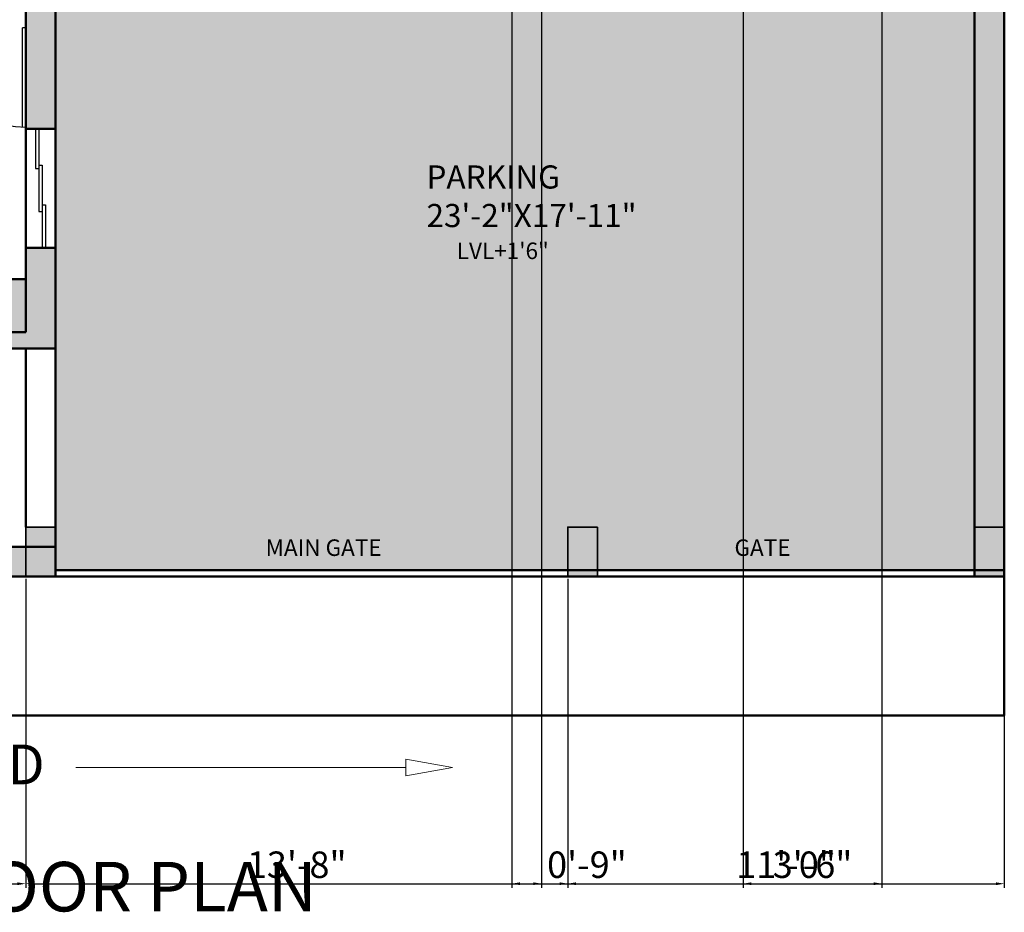
# Model space of a CAD drawing. Units: inches. Extents: x 1770 to 3141, y 984 to 1614.
# Tile 5 of 12: x 2115 to 2413, y 984 to 1254. Entities that reach past the tile are written whole.
import ezdxf

# ---------------------------------------------------------------- set-up
doc = ezdxf.new("R2010")
doc.units = ezdxf.units.IN
for name, color, linetype, lineweight in [('A-ANNO-DIMS', 2, 'Continuous', 18), ('A-ANNO-SYMB', 7, 'Continuous', 18), ('A-ANNO-TEXT', 7, 'Continuous', 18), ('A-AREA-IDEN', 3, 'Continuous', 18), ('A-COLS', 1, 'Continuous', 35), ('A-DOOR', 4, 'Continuous', 25), ('A-FLOR-PATT', 252, 'Continuous', 13), ('A-GLAZ', 5, 'Continuous', 25), ('A-WALL', 7, 'Continuous', 50), ('A-WALL-PATT', 8, 'Continuous', 13)]:
    doc.layers.add(name, color=color, linetype=linetype, lineweight=lineweight)
doc.styles.get("Standard").update_dxf_attribs({"font": 'arial.ttf'})
doc.dimstyles.new('ISO-25', dxfattribs={"dimtxt": 8, "dimasz": 2.5, "dimexe": 1.25, "dimexo": 0.625, "dimtad": 1, "dimdec": 1, "dimlunit": 3, "dimtxsty": 'Standard', "dimcen": 2.5, "dimclrt": 1, "dimadec": 0, "dimazin": 0, "dimtfac": 1, "dimtdec": 1, "dimtmove": 0, "dimatfit": 3, "dimfxl": 1, "dimarcsym": 0})

# ---------------------------------------------------------------- blocks, each defined once
blk = doc.blocks.new("D2 2'6")
for p, q in [((0, 30), (0, 0)), ((1, 30), (1, 0)), ((0, 0), (1, 0))]:
    blk.add_line(p, q)
blk.add_arc((0, 0), 30, 0, 90)
blk = doc.blocks.new('COLUMN-9x15')
at = {"transparency": 33554687}
h = blk.add_hatch(color=256, dxfattribs=at)
h.dxf.hatch_style = 1
h.paths.add_polyline_path([(9, 15), (0, 15), (0, 0), (9, 0)])
blk.add_lwpolyline([(9, 15), (0, 15), (0, 0), (9, 0)], close=True)
blk = doc.blocks.new('*D111')
at = {"layer": 'A-ANNO-DIMS', "color": 0, "lineweight": -2, "transparency": 16777216}
for p, q in [((2001.73, 1084.55), (2001.73, 991.02)), ((2116.73, 1084.55), (2116.73, 991.02)), ((2004.23, 992.27), (2114.23, 992.27))]:
    blk.add_line(p, q, dxfattribs=at)
at = {"layer": 'A-ANNO-DIMS', "color": 0, "transparency": 16777216}
for points in [[(2004.23, 992.69), (2004.23, 991.85), (2001.73, 992.27)], [(2114.23, 992.69), (2114.23, 991.85), (2116.73, 992.27)]]:
    blk.add_solid(points, dxfattribs=at)
at = {"layer": 'Defpoints', "color": 0, "transparency": 16777216}
for p in [(2001.73, 1085.18), (2116.73, 1085.18), (2116.73, 992.27)]:
    blk.add_point(p, dxfattribs=at)
at = {"layer": 'A-ANNO-DIMS', "color": 1, "transparency": 16777216, "insert": (2059.23, 996.98), "char_height": 8, "attachment_point": 5}
blk.add_mtext('9\'-7"', dxfattribs=at)
blk = doc.blocks.new('*D112')
at = {"layer": 'A-ANNO-DIMS', "color": 0, "lineweight": -2, "transparency": 16777216}
for p, q in [((2116.73, 1084.55), (2116.73, 991.02)), ((2280.7, 1084.55), (2280.7, 991.02)), ((2119.23, 992.27), (2278.2, 992.27))]:
    blk.add_line(p, q, dxfattribs=at)
at = {"layer": 'A-ANNO-DIMS', "color": 0, "transparency": 16777216}
for points in [[(2119.23, 992.69), (2119.23, 991.85), (2116.73, 992.27)], [(2278.2, 992.69), (2278.2, 991.85), (2280.7, 992.27)]]:
    blk.add_solid(points, dxfattribs=at)
at = {"layer": 'Defpoints', "color": 0, "transparency": 16777216}
for p in [(2116.73, 1085.18), (2280.7, 1085.18), (2280.7, 992.27)]:
    blk.add_point(p, dxfattribs=at)
at = {"layer": 'A-ANNO-DIMS', "color": 1, "transparency": 16777216, "insert": (2198.71, 996.98), "char_height": 8, "attachment_point": 5}
blk.add_mtext('13\'-8"', dxfattribs=at)
blk = doc.blocks.new('*D113')
at = {"layer": 'A-ANNO-DIMS', "color": 0, "lineweight": -2, "transparency": 16777216}
for p, q in [((2280.7, 1084.55), (2280.7, 991.02)), ((2412.73, 1084.55), (2412.73, 991.02)), ((2283.2, 992.27), (2410.23, 992.27))]:
    blk.add_line(p, q, dxfattribs=at)
at = {"layer": 'A-ANNO-DIMS', "color": 0, "transparency": 16777216}
for points in [[(2283.2, 992.69), (2283.2, 991.85), (2280.7, 992.27)], [(2410.23, 992.69), (2410.23, 991.85), (2412.73, 992.27)]]:
    blk.add_solid(points, dxfattribs=at)
at = {"layer": 'Defpoints', "color": 0, "transparency": 16777216}
for p in [(2280.7, 1085.18), (2412.73, 1085.18), (2412.73, 992.27)]:
    blk.add_point(p, dxfattribs=at)
at = {"layer": 'A-ANNO-DIMS', "color": 1, "transparency": 16777216, "insert": (2346.71, 996.98), "char_height": 8, "attachment_point": 5}
blk.add_mtext('11\'-0"', dxfattribs=at)
blk = doc.blocks.new('*D118')
at = {"layer": 'A-ANNO-DIMS', "color": 0, "lineweight": -2, "transparency": 16777216}
for p, q in [((2272.73, 1355.55), (2272.73, 991.02)), ((2263.73, 1346.55), (2263.73, 991.02)), ((2266.23, 992.27), (2270.23, 992.27)), ((2272.73, 992.27), (2297.75, 992.27))]:
    blk.add_line(p, q, dxfattribs=at)
at = {"layer": 'A-ANNO-DIMS', "color": 0, "transparency": 16777216}
for points in [[(2266.23, 992.69), (2266.23, 991.85), (2263.73, 992.27)], [(2270.23, 992.69), (2270.23, 991.85), (2272.73, 992.27)]]:
    blk.add_solid(points, dxfattribs=at)
at = {"layer": 'Defpoints', "color": 0, "transparency": 16777216}
for p in [(2272.73, 1356.18), (2263.73, 1347.18), (2272.73, 992.27)]:
    blk.add_point(p, dxfattribs=at)
at = {"layer": 'A-ANNO-DIMS', "color": 1, "transparency": 16777216, "insert": (2286.49, 996.98), "char_height": 8, "attachment_point": 5}
blk.add_mtext('0\'-9"', dxfattribs=at)
blk = doc.blocks.new('*D119')
at = {"layer": 'A-ANNO-DIMS', "color": 0, "lineweight": -2, "transparency": 16777216}
for p, q in [((2333.73, 1355.55), (2333.73, 991.02)), ((2375.73, 1346.55), (2375.73, 991.02)), ((2336.23, 992.27), (2373.23, 992.27))]:
    blk.add_line(p, q, dxfattribs=at)
at = {"layer": 'A-ANNO-DIMS', "color": 0, "transparency": 16777216}
for points in [[(2336.23, 992.69), (2336.23, 991.85), (2333.73, 992.27)], [(2373.23, 992.69), (2373.23, 991.85), (2375.73, 992.27)]]:
    blk.add_solid(points, dxfattribs=at)
at = {"layer": 'Defpoints', "color": 0, "transparency": 16777216}
for p in [(2333.73, 1356.18), (2375.73, 1347.18), (2375.73, 992.27)]:
    blk.add_point(p, dxfattribs=at)
at = {"layer": 'A-ANNO-DIMS', "color": 1, "transparency": 16777216, "insert": (2354.73, 996.98), "char_height": 8, "attachment_point": 5}
blk.add_mtext('3\'-6"', dxfattribs=at)

msp = doc.modelspace()

# ---------------------------------------------------------------- hatches: boundary and pattern name
at = {"layer": 'A-FLOR-PATT'}
h = msp.add_hatch(color=256, dxfattribs=at)
h.dxf.hatch_style = 1
h.paths.add_polyline_path([(2403.73, 1288.18), (2239.73, 1288.18), (2239.73, 1300.18), (2193.73, 1300.18), (2193.73, 1288.18), (2125.73, 1288.18), (2125.73, 1154.18), (2125.73, 1087.18), (2280.7, 1087.18), (2280.7, 1100.18), (2289.7, 1100.18), (2289.7, 1087.18), (2403.73, 1087.18), (2403.73, 1100.18)])
h.paths.add_polyline_path([(2235.45, 1177.86), (2301.2, 1177.86), (2301.2, 1213.08), (2235.45, 1213.08)], flags=24)
h.paths.add_polyline_path([(2328.34, 1088.62), (2351.8, 1088.62), (2351.8, 1098.92), (2328.34, 1098.92)], flags=24)
h.paths.add_polyline_path([(2187.53, 1088.62), (2228.45, 1088.62), (2228.45, 1098.92), (2187.53, 1098.92)], flags=24)
at = {"layer": 'A-WALL-PATT'}
h = msp.add_hatch(color=256, dxfattribs=at)
h.dxf.hatch_style = 1
h.paths.add_polyline_path([(1821.73, 1556.18), (1844.25, 1556.18), (2086.73, 1556.18), (2086.73, 1443.18), (2091.73, 1443.18), (2091.73, 1556.18), (2239.73, 1556.18), (2239.73, 1565.18), (1812.73, 1565.18), (1812.73, 1100.18), (1821.73, 1100.18), (1821.73, 1246.18), (1913.73, 1246.18), (1913.73, 1251.18), (1821.73, 1251.18), (1821.73, 1407.18), (1944.73, 1407.18), (1944.73, 1412.18), (1821.73, 1412.18)])
h.paths.add_polyline_path([(1985.73, 1515.18), (1997.73, 1515.18), (1997.73, 1520.18), (1980.73, 1520.18), (1980.73, 1478.18), (1985.73, 1478.18)], flags=16)
h.paths.add_polyline_path([(2038.73, 1520.18), (2021.73, 1520.18), (2021.73, 1515.18), (2033.73, 1515.18), (2033.73, 1412.18), (1985.73, 1412.18), (1985.73, 1448.18), (1980.73, 1448.18), (1980.73, 1407.18), (2038.73, 1407.18), (2038.73, 1443.18), (2056.73, 1443.18), (2056.73, 1448.18), (2038.73, 1448.18)], flags=17)
h.paths.add_polyline_path([(1853.23, 1094.18), (1821.73, 1094.18), (1821.73, 1085.18), (1853.23, 1085.18)])
h.paths.add_polyline_path([(2001.73, 1094.18), (1966.73, 1094.18), (1966.73, 1124.18), (1961.73, 1124.18), (1961.73, 1094.18), (1889.23, 1094.18), (1889.23, 1085.18), (2001.73, 1085.18)])
h.paths.add_polyline_path([(2020.69, 1094.18), (2010.73, 1094.18), (2010.73, 1085.18), (2020.69, 1085.18)])
h.paths.add_polyline_path([(2116.73, 1094.18), (2080.69, 1094.18), (2080.69, 1085.18), (2116.73, 1085.18)])
h.paths.add_polyline_path([(2125.73, 1184.68), (2116.73, 1184.68), (2116.73, 1159.18), (2056.73, 1159.18), (2056.73, 1246.18), (2086.73, 1246.18), (2086.73, 1251.18), (2001.73, 1251.18), (2001.73, 1246.18), (2051.73, 1246.18), (2051.73, 1159.18), (1966.73, 1159.18), (1966.73, 1246.18), (1971.73, 1246.18), (1971.73, 1251.18), (1961.73, 1251.18), (1961.73, 1154.18), (1991.73, 1154.18), (2125.73, 1154.18)], flags=17)
h.paths.add_polyline_path([(2125.73, 1256.18), (2116.73, 1256.18), (2116.73, 1220.68), (2125.73, 1220.68)], flags=17)
h.paths.add_polyline_path([(2128.73, 1309.18), (2116.73, 1309.18), (2116.73, 1292.18), (2125.73, 1292.18), (2125.73, 1300.18), (2128.73, 1300.18)], flags=17)
h.paths.add_polyline_path([(2239.73, 1309.18), (2217.73, 1309.18), (2217.73, 1300.18), (2239.73, 1300.18)], flags=17)
h.paths.add_polyline_path([(2181.73, 1309.18), (2176.73, 1309.18), (2176.73, 1300.18), (2181.73, 1300.18)], flags=17)
h = msp.add_hatch(color=256, dxfattribs=at)
h.dxf.hatch_style = 1
h.paths.add_polyline_path([(2412.73, 1300.18), (2403.73, 1300.18), (2403.73, 1100.18), (2412.73, 1100.18)])
h = msp.add_hatch(color=256, dxfattribs=at)
h.dxf.hatch_style = 1
h.paths.add_polyline_path([(2116.73, 1175.18), (2056.73, 1175.18), (2056.73, 1159.18), (2116.73, 1159.18)])

# ---------------------------------------------------------------- linework, layer by layer
at = {"layer": 'A-ANNO-SYMB'}
msp.add_line((2231.68, 1027.42), (2131.87, 1027.42), dxfattribs=at)
msp.add_lwpolyline([(2245.84, 1027.42), (2231.68, 1029.98), (2231.68, 1024.87)], close=True, dxfattribs=at)
at = {"layer": 'A-GLAZ'}
for p, q in [((2119.73, 1220.68), (2119.73, 1208.68)), ((2120.73, 1220.68), (2120.73, 1195.68)), ((2120.73, 1209.68), (2121.73, 1209.68)), ((2121.73, 1209.68), (2121.73, 1184.68)), ((2119.73, 1208.68), (2120.73, 1208.68)), ((2121.73, 1197.68), (2122.73, 1197.68)), ((2122.73, 1197.68), (2122.73, 1184.68)), ((2120.73, 1195.68), (2121.73, 1195.68))]:
    msp.add_line(p, q, dxfattribs=at)
at = {"layer": 'A-WALL'}
for p, q in [((2412.73, 1565.18), (2412.73, 1043.18)), ((2116.73, 1159.18), (2116.73, 1309.18)), ((2125.73, 1154.18), (2125.73, 1300.18)), ((2403.73, 1300.18), (2403.73, 1085.18)), ((2116.73, 1220.68), (2125.73, 1220.68)), ((2116.73, 1184.68), (2125.73, 1184.68)), ((2116.73, 1175.18), (2056.73, 1175.18)), ((2116.73, 1159.18), (2056.73, 1159.18)), ((2125.73, 1154.18), (1961.73, 1154.18)), ((2116.73, 1154.18), (2116.73, 1100.18)), ((2125.73, 1154.18), (2125.73, 1085.18)), ((2125.73, 1085.18), (2125.73, 1100.18)), ((2125.73, 1094.18), (1966.73, 1094.18)), ((2412.73, 1087.18), (2125.73, 1087.18)), ((2412.73, 1085.18), (1812.73, 1085.18)), ((2412.73, 1043.18), (1812.73, 1043.18))]:
    msp.add_line(p, q, dxfattribs=at)

# ---------------------------------------------------------------- block references
at = {"layer": 'A-COLS'}
for p in [(2116.73, 1085.18), (2280.7, 1085.18), (2403.73, 1085.18)]:
    msp.add_blockref('COLUMN-9x15', p, dxfattribs=at)
at = {"layer": 'A-DOOR', "rotation": 180}
msp.add_blockref("D2 2'6", (2116.73, 1251.18), dxfattribs=at)

# ---------------------------------------------------------------- texts
at = {"layer": 'A-ANNO-TEXT', "attachment_point": 1}
for s, width, heights, insert, char_height in [('{MAIN GATE}', 86.9528, [5.17], (2189.3, 1096.44), 5), ('{ GATE}', 86.9528, [5.17], (2329.59, 1096.44), 5), ('  ROAD', 86.9528, [0], (2071.39, 1034.35), 12), ('GROUND FLOOR PLAN', 253.2094, [0], (1992.64, 998.88), 15)]:
    msp.add_mtext_dynamic_manual_height_columns(s, width=width, gutter_width=12.5, heights=heights, dxfattribs=dict(at, insert=insert, char_height=char_height))
at = {"layer": 'A-AREA-IDEN', "insert": (2237.95, 1209.59), "char_height": 7, "attachment_point": 1}
msp.add_mtext_dynamic_manual_height_columns('PARKING     23\'-2"X17\'-11"\\P{\\H0.71429x;      LVL+1\'6"}', width=86.9528, gutter_width=12.5, heights=[0], dxfattribs=at)

# ---------------------------------------------------------------- dimensions: what is measured, and where the dimension line sits
at = {"layer": 'A-ANNO-DIMS'}
for base, p1, p2, picture, middle in [((2272.73, 992.27), (2263.73, 1347.18), (2272.73, 1356.18), '*D118', (2286.49, 996.98)), ((2375.73, 992.27), (2333.73, 1356.18), (2375.73, 1347.18), '*D119', (2354.73, 996.98)), ((2116.73, 992.27), (2001.73, 1085.18), (2116.73, 1085.18), '*D111', (2059.23, 996.98)), ((2280.7, 992.27), (2116.73, 1085.18), (2280.7, 1085.18), '*D112', (2198.71, 996.98)), ((2412.73, 992.27), (2280.7, 1085.18), (2412.73, 1085.18), '*D113', (2346.71, 996.98))]:
    dim = msp.add_linear_dim(base=base, p1=p1, p2=p2, dimstyle='ISO-25', override={"dimdec": 1, "dimlfac": 1, "dimrnd": 0, "dimzin": 1, "dimdsep": 46, "dimlunit": 4, "dimfrac": 2}, dxfattribs=at)
    dim.commit()
    dim.dimension.update_dxf_attribs({"geometry": picture, "text_midpoint": middle})

doc.saveas('drawing.dxf')
